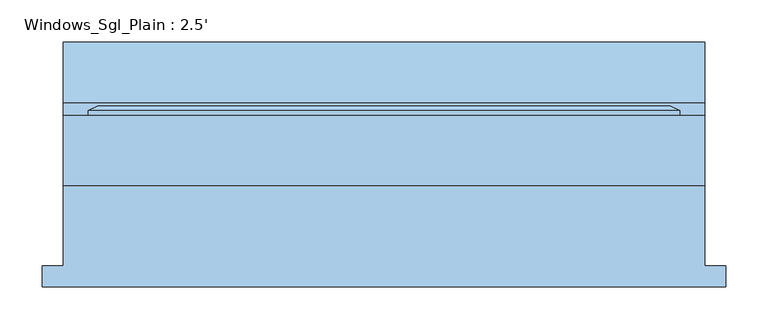
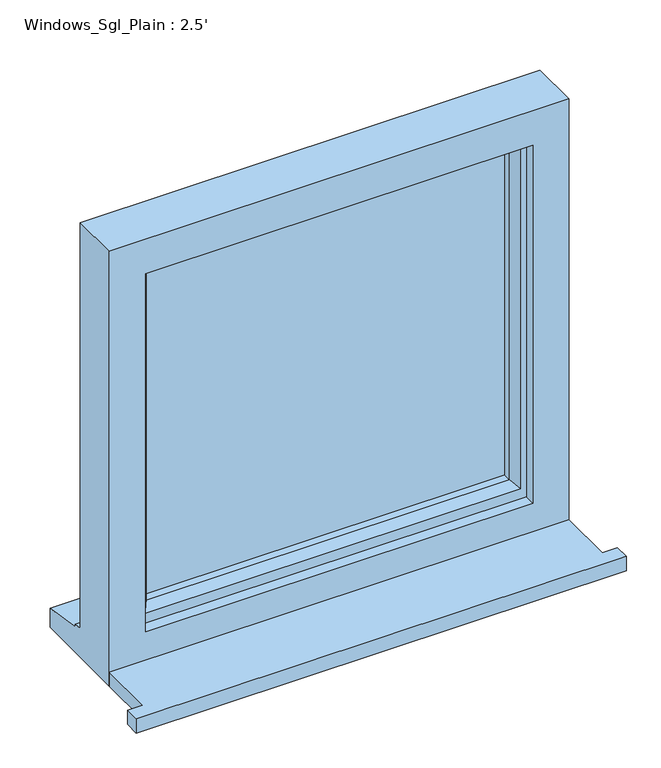
"""IFC4 building model written with IfcOpenShell, lengths in millimetres: window geometry, Windows_Sgl_Plain : 2.5'."""

from ifc_helpers import new_model, si_unit, frame, origin, place, context, project, spatial, polyline, outline, extrude, faceted_brep, source, transform, mapped, element, save


def windows_sgl_plain_2_5_1233c963(model_context):
    return source(origin(), model_context, "Body", "SolidModel", [
        extrude(outline(polyline([(-406.0, -130.8434322), (-406.0, -105.8434322), (-381.0, -105.8434322), (-381.0, -10.2434322), (381.0, -10.2434322), (381.0, -105.8434322), (406.0, -105.8434322), (406.0, -130.8434322), (-406.0, -130.8434322)])), frame((0.0, 0.0, 1348.0), z_axis=(0.0, 0.0, 1.0), x_axis=(1.0, 0.0, 0.0)), (0.0, 0.0, 1.0), 25.0),
        faceted_brep([(-381.0, -10.2434322, 1348.0), (381.0, -10.2434322, 1348.0), (381.0, -10.2434322, 2110.0), (-381.0, -10.2434322, 2110.0), (-321.0, -10.2434322, 2050.0), (321.0, -10.2434322, 2050.0), (321.0, -10.2434322, 1423.0), (-321.0, -10.2434322, 1423.0), (-381.0, 72.7565678, 2110.0), (-381.0, 72.7565678, 1399.0), (-381.0, 87.7565678, 1397.68767), (-381.0, 87.7565678, 1392.7449676), (-381.0, 160.2565678, 1381.8088847), (-381.0, 160.2565678, 1348.0), (381.0, 72.7565678, 2110.0), (381.0, 72.7565678, 1399.0), (-341.0, 72.7565678, 2070.0), (-341.0, 72.7565678, 1411.0), (341.0, 72.7565678, 1411.0), (341.0, 72.7565678, 2070.0), (-341.0, 7.7565678, 2070.0), (-341.0, 7.7565678, 1411.0), (341.0, 7.7565678, 2070.0), (341.0, 7.7565678, 1411.0), (-321.0, 7.7565678, 2050.0), (-321.0, 7.7565678, 1423.0), (321.0, 7.7565678, 1423.0), (321.0, 7.7565678, 2050.0), (381.0, 160.2565678, 1348.0), (381.0, 160.2565678, 1381.8088847), (381.0, 87.7565678, 1392.7449676), (381.0, 87.7565678, 1397.68767)], [[[0, 1, 2, 3], [4, 5, 6, 7]], [[0, 3, 8, 9, 10, 11, 12, 13]], [[9, 8, 14, 15], [16, 17, 18, 19]], [[17, 16, 20, 21]], [[20, 22, 23, 21], [24, 25, 26, 27]], [[24, 4, 7, 25]], [[3, 2, 14, 8]], [[16, 19, 22, 20]], [[5, 4, 24, 27]], [[15, 14, 2, 1, 28, 29, 30, 31]], [[19, 18, 23, 22]], [[5, 27, 26, 6]], [[28, 1, 0, 13]], [[29, 28, 13, 12]], [[30, 29, 12, 11]], [[31, 30, 11, 10]], [[15, 31, 10, 9]], [[21, 23, 18, 17]], [[7, 6, 26, 25]]]),
        extrude(outline(polyline([(311.0, 36.7565678), (-311.0, 36.7565678), (-311.0, 60.7565678), (311.0, 60.7565678), (311.0, 36.7565678)])), frame((0.0, 0.0, 1441.0), z_axis=(0.0, 0.0, 1.0), x_axis=(1.0, 0.0, 0.0)), (0.0, 0.0, 1.0), 599.0),
        faceted_brep([(-351.0, 72.7565678, 2080.0), (-351.0, 78.5300705, 2080.0), (-351.0, 78.5300705, 1401.0), (-351.0, 72.7565678, 1401.0), (-341.0, 7.7565678, 2070.0), (-341.0, 72.7565678, 2070.0), (-341.0, 72.7565678, 1411.0), (-341.0, 7.7565678, 1411.0), (-301.0, 22.2494677, 2030.0), (-311.1480377, 7.7565678, 2040.1480377), (-311.1480377, 7.7565678, 1440.8519623), (-301.0, 22.2494677, 1451.0), (-301.0, 36.7565678, 2030.0), (-301.0, 36.7565678, 1451.0), (-311.0, 60.7565678, 2040.0), (-311.0, 36.7565678, 2040.0), (-311.0, 36.7565678, 1441.0), (-311.0, 60.7565678, 1441.0), (-301.0, 78.5300705, 2030.0), (-301.0, 60.7565678, 2030.0), (-301.0, 60.7565678, 1451.0), (-301.0, 78.5300705, 1451.0), (-318.4457548, 84.3035732, 2047.4457548), (-318.4457548, 84.3035732, 1433.5542452), (-340.2153903, 84.3035732, 2069.2153903), (-340.2153903, 84.3035732, 1411.7846097), (351.0, 78.5300705, 1401.0), (351.0, 72.7565678, 1401.0), (341.0, 72.7565678, 1411.0), (341.0, 7.7565678, 1411.0), (311.1480377, 7.7565678, 1440.8519623), (301.0, 22.2494677, 1451.0), (301.0, 36.7565678, 1451.0), (311.0, 36.7565678, 1441.0), (311.0, 60.7565678, 1441.0), (301.0, 60.7565678, 1451.0), (301.0, 78.5300705, 1451.0), (318.4457548, 84.3035732, 1433.5542452), (340.2153903, 84.3035732, 1411.7846097), (351.0, 78.5300705, 2080.0), (351.0, 72.7565678, 2080.0), (341.0, 72.7565678, 2070.0), (341.0, 7.7565678, 2070.0), (311.1480377, 7.7565678, 2040.1480377), (301.0, 22.2494677, 2030.0), (301.0, 36.7565678, 2030.0), (311.0, 36.7565678, 2040.0), (311.0, 60.7565678, 2040.0), (301.0, 60.7565678, 2030.0), (301.0, 78.5300705, 2030.0), (318.4457548, 84.3035732, 2047.4457548), (340.2153903, 84.3035732, 2069.2153903)], [[[0, 1, 2, 3]], [[4, 5, 6, 7]], [[8, 9, 10, 11]], [[12, 8, 11, 13]], [[14, 15, 16, 17]], [[18, 19, 20, 21]], [[22, 18, 21, 23]], [[1, 24, 25, 2]], [[3, 2, 26, 27]], [[7, 6, 28, 29]], [[11, 10, 30, 31]], [[13, 11, 31, 32]], [[17, 16, 33, 34]], [[21, 20, 35, 36]], [[23, 21, 36, 37]], [[2, 25, 38, 26]], [[27, 26, 39, 40]], [[29, 28, 41, 42]], [[31, 30, 43, 44]], [[32, 31, 44, 45]], [[34, 33, 46, 47]], [[36, 35, 48, 49]], [[37, 36, 49, 50]], [[26, 38, 51, 39]], [[40, 39, 1, 0]], [[3, 27, 40, 0], [5, 41, 28, 6]], [[42, 41, 5, 4]], [[7, 29, 42, 4], [9, 43, 30, 10]], [[44, 43, 9, 8]], [[45, 44, 8, 12]], [[15, 46, 33, 16], [13, 32, 45, 12]], [[47, 46, 15, 14]], [[17, 34, 47, 14], [19, 48, 35, 20]], [[49, 48, 19, 18]], [[50, 49, 18, 22]], [[24, 51, 38, 25], [23, 37, 50, 22]], [[39, 51, 24, 1]]]),
    ])


if __name__ == "__main__":
    model = new_model("IFC4")
    model_context = context("Model", 3, world=origin())
    ifc_project = project(units=[si_unit("LENGTHUNIT", "METRE", prefix="MILLI")], contexts=[model_context])
    site = spatial("IfcSite", under=ifc_project)
    building = spatial("IfcBuilding", under=site)
    placement = place(None, origin())
    windows_sgl_plain_2_5_shape = windows_sgl_plain_2_5_1233c963(model_context)
    element("IfcWindow", 1, ObjectType="Windows_Sgl_Plain : 2.5'", at=placement, inside=building, context=model_context, shape_type="MappedRepresentation", body=[
        mapped(windows_sgl_plain_2_5_shape, transform((0.0, 0.0, 0.0), x_axis=(1.0, 0.0, 0.0), y_axis=(0.0, 1.0, 0.0), z_axis=(0.0, 0.0, 1.0))),
    ])
    save(model, "model.ifc")

# Revit data of these elements
# Type "Windows_Sgl_Plain : 2.5'"
#   Type Mark = "61"
#   Operation = "SinglePanel"
#   Construction Type Id = "SGL"
#   Manufacturer = "Revit"
#   Keynote = "L10"
#   Analytic Construction = "Large single-glazed windows"
#   Wrap Layers (Ext) from Ext = 0.336286 ft
#   Wrap Layers (Int) from Ext = 0.582349 ft
#   Window Board Projection = 0.082021 ft
#   Window Board Extension = 0.082021 ft
#   Visual Light Transmittance = 0.9
#   Solar Heat Gain Coefficient = 0.86
#   Rough Width = 2.5 ft
#   Rough Height = 2.5 ft
#   Height = 2.5 ft
#   Width = 2.5 ft
#   Heat Transfer Coefficient (U) = 5.5617 W/(m²·K)
#   Glazing Thickness = 0.07874 ft
#   FrameOffset - External = 0.164042 ft
#   Frame Depth = 0.213255 ft
#   Default Head Height = 6.922572 ft
#   Cill Depth = 0.287073 ft
#   Cavity Closer Width = 0.164042 ft
#   Cavity Closer Offset from Ext = 0.336286 ft
#   Cavity Closer Depth = 0.278871 ft
#   Vis - Cavity Closers = yes
#   Define Thermal Properties by = 1
#   Material Trim = Window Frame
#   Material Glass = Glass
#   Material Frame = Window Frame
#   Wall Closure = (empty or 0)
# Element 1 (IfcWindow, "Windows_Sgl_Plain : 2.5'")
#   Materials on its faces: "Window Frame", "Glass"
# Materials
#   "Window Frame": colour RGB 249 249 249, transparency 0, Keynote = "L10", Cost = 0
#   "Glass": class "Glass", colour RGB 0 128 192, transparency 0.9, Description = "Soda Lime Glass", Cost = 0
